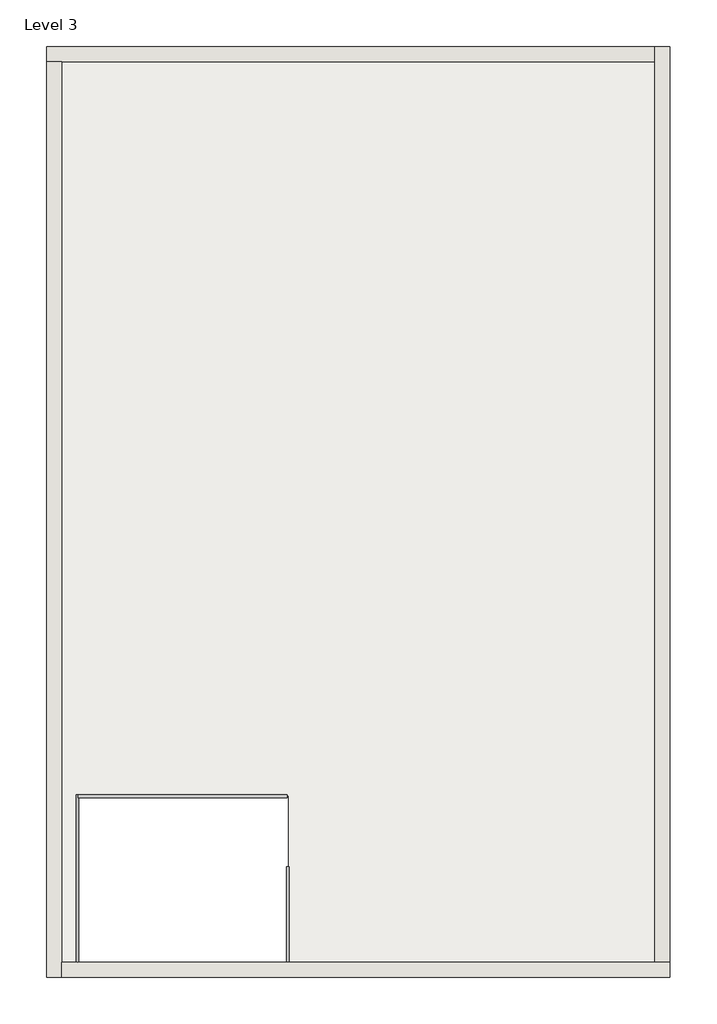
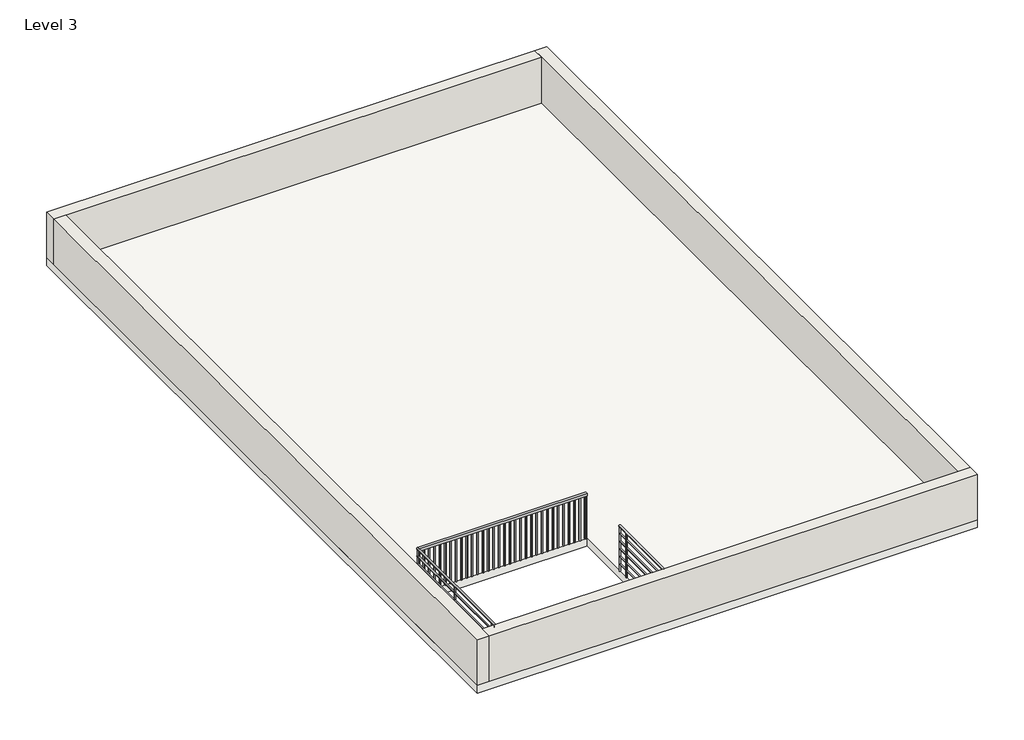
# One storey: 4 walls, 3 railings, 1 slab.
"""IFC4 building model written with IfcOpenShell, lengths in millimetres."""

from ifc_helpers import new_model, si_unit, point, frame, frame_2d, origin, place, context, project, spatial, polyline, circle_curve, trimmed, segment, composite_curve, outline, extrude, faceted_brep, element, save

model = new_model("IFC4")

# Units and contexts
model_context = context("Model", 3, world=origin())
ifc_project = project(units=[si_unit("LENGTHUNIT", "METRE", prefix="MILLI")], contexts=[model_context])

# Site, building, storey
site = spatial("IfcSite", under=ifc_project)
building = spatial("IfcBuilding", under=site)
storey = spatial("IfcBuildingStorey", under=building, Name="Level 3", Elevation=6400.8)

# Railings
placement = place(None, origin())
element("IfcRailing", 1, ObjectType="Handrail - Pipe", at=placement, inside=storey, context=model_context, shape_type="SweptSolid", body=[
    extrude(outline(composite_curve([segment(trimmed(circle_curve(frame_2d((7296.15, -11110.4683044)), 19.05), [point((7296.15, -11129.5183044))], [point((7296.15, -11091.4183044))], False, "CARTESIAN"), True, "CONTINUOUS"), segment(trimmed(circle_curve(frame_2d((7296.15, -11110.4683044)), 19.05), [point((7296.15, -11091.4183044))], [point((7296.15, -11129.5183044))], False, "CARTESIAN"), True, "CONTINUOUS")], self_intersect=False)), frame((0.0, -3889.1891189, 0.0), z_axis=(0.0, 1.0, 0.0), x_axis=(0.0, 0.0, 1.0)), (0.0, 0.0, 1.0), 2540.0),
    extrude(outline(composite_curve([segment(trimmed(circle_curve(frame_2d((7150.1, -11110.4683044)), 12.7), [point((7150.1, -11097.7683044))], [point((7150.1, -11123.1683044))], False, "CARTESIAN"), True, "CONTINUOUS"), segment(trimmed(circle_curve(frame_2d((7150.1, -11110.4683044)), 12.7), [point((7150.1, -11123.1683044))], [point((7150.1, -11097.7683044))], False, "CARTESIAN"), True, "CONTINUOUS")], self_intersect=False)), frame((0.0, -3889.1891189, 0.0), z_axis=(0.0, 1.0, 0.0), x_axis=(0.0, 0.0, 1.0)), (0.0, 0.0, 1.0), 2540.0),
    extrude(outline(composite_curve([segment(trimmed(circle_curve(frame_2d((6997.7, -11110.4683044)), 12.7), [point((6997.7, -11097.7683044))], [point((6997.7, -11123.1683044))], False, "CARTESIAN"), True, "CONTINUOUS"), segment(trimmed(circle_curve(frame_2d((6997.7, -11110.4683044)), 12.7), [point((6997.7, -11123.1683044))], [point((6997.7, -11097.7683044))], False, "CARTESIAN"), True, "CONTINUOUS")], self_intersect=False)), frame((0.0, -3889.1891189, 0.0), z_axis=(0.0, 1.0, 0.0), x_axis=(0.0, 0.0, 1.0)), (0.0, 0.0, 1.0), 2540.0),
    extrude(outline(composite_curve([segment(trimmed(circle_curve(frame_2d((6845.3, -11110.4683044)), 12.7), [point((6845.3, -11097.7683044))], [point((6845.3, -11123.1683044))], False, "CARTESIAN"), True, "CONTINUOUS"), segment(trimmed(circle_curve(frame_2d((6845.3, -11110.4683044)), 12.7), [point((6845.3, -11123.1683044))], [point((6845.3, -11097.7683044))], False, "CARTESIAN"), True, "CONTINUOUS")], self_intersect=False)), frame((0.0, -3889.1891189, 0.0), z_axis=(0.0, 1.0, 0.0), x_axis=(0.0, 0.0, 1.0)), (0.0, 0.0, 1.0), 2540.0),
    extrude(outline(composite_curve([segment(trimmed(circle_curve(frame_2d((6692.9, -11110.4683044)), 12.7), [point((6692.9, -11097.7683044))], [point((6692.9, -11123.1683044))], False, "CARTESIAN"), True, "CONTINUOUS"), segment(trimmed(circle_curve(frame_2d((6692.9, -11110.4683044)), 12.7), [point((6692.9, -11123.1683044))], [point((6692.9, -11097.7683044))], False, "CARTESIAN"), True, "CONTINUOUS")], self_intersect=False)), frame((0.0, -3889.1891189, 0.0), z_axis=(0.0, 1.0, 0.0), x_axis=(0.0, 0.0, 1.0)), (0.0, 0.0, 1.0), 2540.0),
    extrude(outline(composite_curve([segment(trimmed(circle_curve(frame_2d((6540.5, -11110.4683044)), 12.7), [point((6540.5, -11097.7683044))], [point((6540.5, -11123.1683044))], False, "CARTESIAN"), True, "CONTINUOUS"), segment(trimmed(circle_curve(frame_2d((6540.5, -11110.4683044)), 12.7), [point((6540.5, -11123.1683044))], [point((6540.5, -11097.7683044))], False, "CARTESIAN"), True, "CONTINUOUS")], self_intersect=False)), frame((0.0, -3889.1891189, 0.0), z_axis=(0.0, 1.0, 0.0), x_axis=(0.0, 0.0, 1.0)), (0.0, 0.0, 1.0), 2540.0),
    extrude(outline(composite_curve([segment(trimmed(circle_curve(frame_2d((-11110.4683044, -3787.5891189)), 12.7), [point((-11097.7683044, -3787.5891189))], [point((-11123.1683044, -3787.5891189))], False, "CARTESIAN"), True, "CONTINUOUS"), segment(trimmed(circle_curve(frame_2d((-11110.4683044, -3787.5891189)), 12.7), [point((-11123.1683044, -3787.5891189))], [point((-11097.7683044, -3787.5891189))], False, "CARTESIAN"), True, "CONTINUOUS")], self_intersect=False)), frame((0.0, 0.0, 6400.8), z_axis=(0.0, 0.0, 1.0), x_axis=(1.0, 0.0, 0.0)), (0.0, 0.0, 1.0), 876.3),
    extrude(outline(composite_curve([segment(trimmed(circle_curve(frame_2d((-11110.4683044, -2568.3891189)), 12.7), [point((-11097.7683044, -2568.3891189))], [point((-11123.1683044, -2568.3891189))], False, "CARTESIAN"), True, "CONTINUOUS"), segment(trimmed(circle_curve(frame_2d((-11110.4683044, -2568.3891189)), 12.7), [point((-11123.1683044, -2568.3891189))], [point((-11097.7683044, -2568.3891189))], False, "CARTESIAN"), True, "CONTINUOUS")], self_intersect=False)), frame((0.0, 0.0, 6400.8), z_axis=(0.0, 0.0, 1.0), x_axis=(1.0, 0.0, 0.0)), (0.0, 0.0, 1.0), 876.3),
    extrude(outline(composite_curve([segment(trimmed(circle_curve(frame_2d((-11110.4683044, -3876.4891189)), 12.7), [point((-11097.7683044, -3876.4891189))], [point((-11123.1683044, -3876.4891189))], False, "CARTESIAN"), True, "CONTINUOUS"), segment(trimmed(circle_curve(frame_2d((-11110.4683044, -3876.4891189)), 12.7), [point((-11123.1683044, -3876.4891189))], [point((-11097.7683044, -3876.4891189))], False, "CARTESIAN"), True, "CONTINUOUS")], self_intersect=False)), frame((0.0, 0.0, 6400.8), z_axis=(0.0, 0.0, 1.0), x_axis=(1.0, 0.0, 0.0)), (0.0, 0.0, 1.0), 876.3),
    extrude(outline(composite_curve([segment(trimmed(circle_curve(frame_2d((-11110.4683044, -1361.8891189)), 12.7), [point((-11097.7683044, -1361.8891189))], [point((-11123.1683044, -1361.8891189))], False, "CARTESIAN"), True, "CONTINUOUS"), segment(trimmed(circle_curve(frame_2d((-11110.4683044, -1361.8891189)), 12.7), [point((-11123.1683044, -1361.8891189))], [point((-11097.7683044, -1361.8891189))], False, "CARTESIAN"), True, "CONTINUOUS")], self_intersect=False)), frame((0.0, 0.0, 6400.8), z_axis=(0.0, 0.0, 1.0), x_axis=(1.0, 0.0, 0.0)), (0.0, 0.0, 1.0), 876.3),
])
element("IfcRailing", 2, ObjectType="Handrail - Pipe", at=placement, inside=storey, context=model_context, shape_type="SweptSolid", body=[
    extrude(outline(composite_curve([segment(trimmed(circle_curve(frame_2d((7296.15, -7922.7683044)), 19.05), [point((7296.15, -7903.7183044))], [point((7296.15, -7941.8183044))], False, "CARTESIAN"), True, "CONTINUOUS"), segment(trimmed(circle_curve(frame_2d((7296.15, -7922.7683044)), 19.05), [point((7296.15, -7941.8183044))], [point((7296.15, -7903.7183044))], False, "CARTESIAN"), True, "CONTINUOUS")], self_intersect=False)), frame((0.0, -3889.1891189, 0.0), z_axis=(0.0, 1.0, 0.0), x_axis=(0.0, 0.0, 1.0)), (0.0, 0.0, 1.0), 1447.8),
    extrude(outline(composite_curve([segment(trimmed(circle_curve(frame_2d((7150.1, -7922.7683044)), 12.7), [point((7150.1, -7935.4683044))], [point((7150.1, -7910.0683044))], False, "CARTESIAN"), True, "CONTINUOUS"), segment(trimmed(circle_curve(frame_2d((7150.1, -7922.7683044)), 12.7), [point((7150.1, -7910.0683044))], [point((7150.1, -7935.4683044))], False, "CARTESIAN"), True, "CONTINUOUS")], self_intersect=False)), frame((0.0, -3889.1891189, 0.0), z_axis=(0.0, 1.0, 0.0), x_axis=(0.0, 0.0, 1.0)), (0.0, 0.0, 1.0), 1447.8),
    extrude(outline(composite_curve([segment(trimmed(circle_curve(frame_2d((6997.7, -7922.7683044)), 12.7), [point((6997.7, -7935.4683044))], [point((6997.7, -7910.0683044))], False, "CARTESIAN"), True, "CONTINUOUS"), segment(trimmed(circle_curve(frame_2d((6997.7, -7922.7683044)), 12.7), [point((6997.7, -7910.0683044))], [point((6997.7, -7935.4683044))], False, "CARTESIAN"), True, "CONTINUOUS")], self_intersect=False)), frame((0.0, -3889.1891189, 0.0), z_axis=(0.0, 1.0, 0.0), x_axis=(0.0, 0.0, 1.0)), (0.0, 0.0, 1.0), 1447.8),
    extrude(outline(composite_curve([segment(trimmed(circle_curve(frame_2d((6845.3, -7922.7683044)), 12.7), [point((6845.3, -7935.4683044))], [point((6845.3, -7910.0683044))], False, "CARTESIAN"), True, "CONTINUOUS"), segment(trimmed(circle_curve(frame_2d((6845.3, -7922.7683044)), 12.7), [point((6845.3, -7910.0683044))], [point((6845.3, -7935.4683044))], False, "CARTESIAN"), True, "CONTINUOUS")], self_intersect=False)), frame((0.0, -3889.1891189, 0.0), z_axis=(0.0, 1.0, 0.0), x_axis=(0.0, 0.0, 1.0)), (0.0, 0.0, 1.0), 1447.8),
    extrude(outline(composite_curve([segment(trimmed(circle_curve(frame_2d((6692.9, -7922.7683044)), 12.7), [point((6692.9, -7935.4683044))], [point((6692.9, -7910.0683044))], False, "CARTESIAN"), True, "CONTINUOUS"), segment(trimmed(circle_curve(frame_2d((6692.9, -7922.7683044)), 12.7), [point((6692.9, -7910.0683044))], [point((6692.9, -7935.4683044))], False, "CARTESIAN"), True, "CONTINUOUS")], self_intersect=False)), frame((0.0, -3889.1891189, 0.0), z_axis=(0.0, 1.0, 0.0), x_axis=(0.0, 0.0, 1.0)), (0.0, 0.0, 1.0), 1447.8),
    extrude(outline(composite_curve([segment(trimmed(circle_curve(frame_2d((6540.5, -7922.7683044)), 12.7), [point((6540.5, -7935.4683044))], [point((6540.5, -7910.0683044))], False, "CARTESIAN"), True, "CONTINUOUS"), segment(trimmed(circle_curve(frame_2d((6540.5, -7922.7683044)), 12.7), [point((6540.5, -7910.0683044))], [point((6540.5, -7935.4683044))], False, "CARTESIAN"), True, "CONTINUOUS")], self_intersect=False)), frame((0.0, -3889.1891189, 0.0), z_axis=(0.0, 1.0, 0.0), x_axis=(0.0, 0.0, 1.0)), (0.0, 0.0, 1.0), 1447.8),
    extrude(outline(composite_curve([segment(trimmed(circle_curve(frame_2d((-7922.7683044, -2669.9891189)), 12.7), [point((-7935.4683044, -2669.9891189))], [point((-7910.0683044, -2669.9891189))], False, "CARTESIAN"), True, "CONTINUOUS"), segment(trimmed(circle_curve(frame_2d((-7922.7683044, -2669.9891189)), 12.7), [point((-7910.0683044, -2669.9891189))], [point((-7935.4683044, -2669.9891189))], False, "CARTESIAN"), True, "CONTINUOUS")], self_intersect=False)), frame((0.0, 0.0, 6400.8), z_axis=(0.0, 0.0, 1.0), x_axis=(1.0, 0.0, 0.0)), (0.0, 0.0, 1.0), 876.3),
    extrude(outline(composite_curve([segment(trimmed(circle_curve(frame_2d((-7922.7683044, -2454.0891189)), 12.7), [point((-7935.4683044, -2454.0891189))], [point((-7910.0683044, -2454.0891189))], False, "CARTESIAN"), True, "CONTINUOUS"), segment(trimmed(circle_curve(frame_2d((-7922.7683044, -2454.0891189)), 12.7), [point((-7910.0683044, -2454.0891189))], [point((-7935.4683044, -2454.0891189))], False, "CARTESIAN"), True, "CONTINUOUS")], self_intersect=False)), frame((0.0, 0.0, 6400.8), z_axis=(0.0, 0.0, 1.0), x_axis=(1.0, 0.0, 0.0)), (0.0, 0.0, 1.0), 876.3),
    extrude(outline(composite_curve([segment(trimmed(circle_curve(frame_2d((-7922.7683044, -3876.4891189)), 12.7), [point((-7935.4683044, -3876.4891189))], [point((-7910.0683044, -3876.4891189))], False, "CARTESIAN"), True, "CONTINUOUS"), segment(trimmed(circle_curve(frame_2d((-7922.7683044, -3876.4891189)), 12.7), [point((-7910.0683044, -3876.4891189))], [point((-7935.4683044, -3876.4891189))], False, "CARTESIAN"), True, "CONTINUOUS")], self_intersect=False)), frame((0.0, 0.0, 6400.8), z_axis=(0.0, 0.0, 1.0), x_axis=(1.0, 0.0, 0.0)), (0.0, 0.0, 1.0), 876.3),
])
element("IfcRailing", 3, ObjectType="Handrail - Rectangular", at=placement, inside=storey, context=model_context, shape_type="SweptSolid", body=[
    extrude(outline(polyline([(-11110.4683044, -1399.9891189), (-11110.4683044, -1349.1891189), (-7935.4683044, -1349.1891189), (-7935.4683044, -1399.9891189), (-11110.4683044, -1399.9891189)])), frame((0.0, 0.0, 7264.4), z_axis=(0.0, 0.0, 1.0), x_axis=(1.0, 0.0, 0.0)), (0.0, 0.0, 1.0), 50.8),
    extrude(outline(polyline([(-7970.3933044, -1384.1141189), (-7970.3933044, -1365.0641189), (-7951.3433044, -1365.0641189), (-7951.3433044, -1384.1141189), (-7970.3933044, -1384.1141189)])), frame((0.0, 0.0, 6400.8), z_axis=(0.0, 0.0, 1.0), x_axis=(1.0, 0.0, 0.0)), (0.0, 0.0, 1.0), 863.6),
    extrude(outline(polyline([(-8071.9933044, -1384.1141189), (-8071.9933044, -1365.0641189), (-8052.9433044, -1365.0641189), (-8052.9433044, -1384.1141189), (-8071.9933044, -1384.1141189)])), frame((0.0, 0.0, 6400.8), z_axis=(0.0, 0.0, 1.0), x_axis=(1.0, 0.0, 0.0)), (0.0, 0.0, 1.0), 863.6),
    extrude(outline(polyline([(-8173.5933044, -1384.1141189), (-8173.5933044, -1365.0641189), (-8154.5433044, -1365.0641189), (-8154.5433044, -1384.1141189), (-8173.5933044, -1384.1141189)])), frame((0.0, 0.0, 6400.8), z_axis=(0.0, 0.0, 1.0), x_axis=(1.0, 0.0, 0.0)), (0.0, 0.0, 1.0), 863.6),
    extrude(outline(polyline([(-8275.1933044, -1384.1141189), (-8275.1933044, -1365.0641189), (-8256.1433044, -1365.0641189), (-8256.1433044, -1384.1141189), (-8275.1933044, -1384.1141189)])), frame((0.0, 0.0, 6400.8), z_axis=(0.0, 0.0, 1.0), x_axis=(1.0, 0.0, 0.0)), (0.0, 0.0, 1.0), 863.6),
    extrude(outline(polyline([(-8376.7933044, -1384.1141189), (-8376.7933044, -1365.0641189), (-8357.7433044, -1365.0641189), (-8357.7433044, -1384.1141189), (-8376.7933044, -1384.1141189)])), frame((0.0, 0.0, 6400.8), z_axis=(0.0, 0.0, 1.0), x_axis=(1.0, 0.0, 0.0)), (0.0, 0.0, 1.0), 863.6),
    extrude(outline(polyline([(-8478.3933044, -1384.1141189), (-8478.3933044, -1365.0641189), (-8459.3433044, -1365.0641189), (-8459.3433044, -1384.1141189), (-8478.3933044, -1384.1141189)])), frame((0.0, 0.0, 6400.8), z_axis=(0.0, 0.0, 1.0), x_axis=(1.0, 0.0, 0.0)), (0.0, 0.0, 1.0), 863.6),
    extrude(outline(polyline([(-8579.9933044, -1384.1141189), (-8579.9933044, -1365.0641189), (-8560.9433044, -1365.0641189), (-8560.9433044, -1384.1141189), (-8579.9933044, -1384.1141189)])), frame((0.0, 0.0, 6400.8), z_axis=(0.0, 0.0, 1.0), x_axis=(1.0, 0.0, 0.0)), (0.0, 0.0, 1.0), 863.6),
    extrude(outline(polyline([(-8681.5933044, -1384.1141189), (-8681.5933044, -1365.0641189), (-8662.5433044, -1365.0641189), (-8662.5433044, -1384.1141189), (-8681.5933044, -1384.1141189)])), frame((0.0, 0.0, 6400.8), z_axis=(0.0, 0.0, 1.0), x_axis=(1.0, 0.0, 0.0)), (0.0, 0.0, 1.0), 863.6),
    extrude(outline(polyline([(-8783.1933044, -1384.1141189), (-8783.1933044, -1365.0641189), (-8764.1433044, -1365.0641189), (-8764.1433044, -1384.1141189), (-8783.1933044, -1384.1141189)])), frame((0.0, 0.0, 6400.8), z_axis=(0.0, 0.0, 1.0), x_axis=(1.0, 0.0, 0.0)), (0.0, 0.0, 1.0), 863.6),
    extrude(outline(polyline([(-8884.7933044, -1384.1141189), (-8884.7933044, -1365.0641189), (-8865.7433044, -1365.0641189), (-8865.7433044, -1384.1141189), (-8884.7933044, -1384.1141189)])), frame((0.0, 0.0, 6400.8), z_axis=(0.0, 0.0, 1.0), x_axis=(1.0, 0.0, 0.0)), (0.0, 0.0, 1.0), 863.6),
    extrude(outline(polyline([(-8986.3933044, -1384.1141189), (-8986.3933044, -1365.0641189), (-8967.3433044, -1365.0641189), (-8967.3433044, -1384.1141189), (-8986.3933044, -1384.1141189)])), frame((0.0, 0.0, 6400.8), z_axis=(0.0, 0.0, 1.0), x_axis=(1.0, 0.0, 0.0)), (0.0, 0.0, 1.0), 863.6),
    extrude(outline(polyline([(-9087.9933044, -1384.1141189), (-9087.9933044, -1365.0641189), (-9068.9433044, -1365.0641189), (-9068.9433044, -1384.1141189), (-9087.9933044, -1384.1141189)])), frame((0.0, 0.0, 6400.8), z_axis=(0.0, 0.0, 1.0), x_axis=(1.0, 0.0, 0.0)), (0.0, 0.0, 1.0), 863.6),
    extrude(outline(polyline([(-9189.5933044, -1384.1141189), (-9189.5933044, -1365.0641189), (-9170.5433044, -1365.0641189), (-9170.5433044, -1384.1141189), (-9189.5933044, -1384.1141189)])), frame((0.0, 0.0, 6400.8), z_axis=(0.0, 0.0, 1.0), x_axis=(1.0, 0.0, 0.0)), (0.0, 0.0, 1.0), 863.6),
    extrude(outline(polyline([(-9291.1933044, -1384.1141189), (-9291.1933044, -1365.0641189), (-9272.1433044, -1365.0641189), (-9272.1433044, -1384.1141189), (-9291.1933044, -1384.1141189)])), frame((0.0, 0.0, 6400.8), z_axis=(0.0, 0.0, 1.0), x_axis=(1.0, 0.0, 0.0)), (0.0, 0.0, 1.0), 863.6),
    extrude(outline(polyline([(-9392.7933044, -1384.1141189), (-9392.7933044, -1365.0641189), (-9373.7433044, -1365.0641189), (-9373.7433044, -1384.1141189), (-9392.7933044, -1384.1141189)])), frame((0.0, 0.0, 6400.8), z_axis=(0.0, 0.0, 1.0), x_axis=(1.0, 0.0, 0.0)), (0.0, 0.0, 1.0), 863.6),
    extrude(outline(polyline([(-9494.3933044, -1384.1141189), (-9494.3933044, -1365.0641189), (-9475.3433044, -1365.0641189), (-9475.3433044, -1384.1141189), (-9494.3933044, -1384.1141189)])), frame((0.0, 0.0, 6400.8), z_axis=(0.0, 0.0, 1.0), x_axis=(1.0, 0.0, 0.0)), (0.0, 0.0, 1.0), 863.6),
    extrude(outline(polyline([(-9595.9933044, -1384.1141189), (-9595.9933044, -1365.0641189), (-9576.9433044, -1365.0641189), (-9576.9433044, -1384.1141189), (-9595.9933044, -1384.1141189)])), frame((0.0, 0.0, 6400.8), z_axis=(0.0, 0.0, 1.0), x_axis=(1.0, 0.0, 0.0)), (0.0, 0.0, 1.0), 863.6),
    extrude(outline(polyline([(-9697.5933044, -1384.1141189), (-9697.5933044, -1365.0641189), (-9678.5433044, -1365.0641189), (-9678.5433044, -1384.1141189), (-9697.5933044, -1384.1141189)])), frame((0.0, 0.0, 6400.8), z_axis=(0.0, 0.0, 1.0), x_axis=(1.0, 0.0, 0.0)), (0.0, 0.0, 1.0), 863.6),
    extrude(outline(polyline([(-9799.1933044, -1384.1141189), (-9799.1933044, -1365.0641189), (-9780.1433044, -1365.0641189), (-9780.1433044, -1384.1141189), (-9799.1933044, -1384.1141189)])), frame((0.0, 0.0, 6400.8), z_axis=(0.0, 0.0, 1.0), x_axis=(1.0, 0.0, 0.0)), (0.0, 0.0, 1.0), 863.6),
    extrude(outline(polyline([(-9900.7933044, -1384.1141189), (-9900.7933044, -1365.0641189), (-9881.7433044, -1365.0641189), (-9881.7433044, -1384.1141189), (-9900.7933044, -1384.1141189)])), frame((0.0, 0.0, 6400.8), z_axis=(0.0, 0.0, 1.0), x_axis=(1.0, 0.0, 0.0)), (0.0, 0.0, 1.0), 863.6),
    extrude(outline(polyline([(-10002.3933044, -1384.1141189), (-10002.3933044, -1365.0641189), (-9983.3433044, -1365.0641189), (-9983.3433044, -1384.1141189), (-10002.3933044, -1384.1141189)])), frame((0.0, 0.0, 6400.8), z_axis=(0.0, 0.0, 1.0), x_axis=(1.0, 0.0, 0.0)), (0.0, 0.0, 1.0), 863.6),
    extrude(outline(polyline([(-10103.9933044, -1384.1141189), (-10103.9933044, -1365.0641189), (-10084.9433044, -1365.0641189), (-10084.9433044, -1384.1141189), (-10103.9933044, -1384.1141189)])), frame((0.0, 0.0, 6400.8), z_axis=(0.0, 0.0, 1.0), x_axis=(1.0, 0.0, 0.0)), (0.0, 0.0, 1.0), 863.6),
    extrude(outline(polyline([(-10205.5933044, -1384.1141189), (-10205.5933044, -1365.0641189), (-10186.5433044, -1365.0641189), (-10186.5433044, -1384.1141189), (-10205.5933044, -1384.1141189)])), frame((0.0, 0.0, 6400.8), z_axis=(0.0, 0.0, 1.0), x_axis=(1.0, 0.0, 0.0)), (0.0, 0.0, 1.0), 863.6),
    extrude(outline(polyline([(-10307.1933044, -1384.1141189), (-10307.1933044, -1365.0641189), (-10288.1433044, -1365.0641189), (-10288.1433044, -1384.1141189), (-10307.1933044, -1384.1141189)])), frame((0.0, 0.0, 6400.8), z_axis=(0.0, 0.0, 1.0), x_axis=(1.0, 0.0, 0.0)), (0.0, 0.0, 1.0), 863.6),
    extrude(outline(polyline([(-10408.7933044, -1384.1141189), (-10408.7933044, -1365.0641189), (-10389.7433044, -1365.0641189), (-10389.7433044, -1384.1141189), (-10408.7933044, -1384.1141189)])), frame((0.0, 0.0, 6400.8), z_axis=(0.0, 0.0, 1.0), x_axis=(1.0, 0.0, 0.0)), (0.0, 0.0, 1.0), 863.6),
    extrude(outline(polyline([(-10510.3933044, -1384.1141189), (-10510.3933044, -1365.0641189), (-10491.3433044, -1365.0641189), (-10491.3433044, -1384.1141189), (-10510.3933044, -1384.1141189)])), frame((0.0, 0.0, 6400.8), z_axis=(0.0, 0.0, 1.0), x_axis=(1.0, 0.0, 0.0)), (0.0, 0.0, 1.0), 863.6),
    extrude(outline(polyline([(-10611.9933044, -1384.1141189), (-10611.9933044, -1365.0641189), (-10592.9433044, -1365.0641189), (-10592.9433044, -1384.1141189), (-10611.9933044, -1384.1141189)])), frame((0.0, 0.0, 6400.8), z_axis=(0.0, 0.0, 1.0), x_axis=(1.0, 0.0, 0.0)), (0.0, 0.0, 1.0), 863.6),
    extrude(outline(polyline([(-10713.5933044, -1384.1141189), (-10713.5933044, -1365.0641189), (-10694.5433044, -1365.0641189), (-10694.5433044, -1384.1141189), (-10713.5933044, -1384.1141189)])), frame((0.0, 0.0, 6400.8), z_axis=(0.0, 0.0, 1.0), x_axis=(1.0, 0.0, 0.0)), (0.0, 0.0, 1.0), 863.6),
    extrude(outline(polyline([(-10815.1933044, -1384.1141189), (-10815.1933044, -1365.0641189), (-10796.1433044, -1365.0641189), (-10796.1433044, -1384.1141189), (-10815.1933044, -1384.1141189)])), frame((0.0, 0.0, 6400.8), z_axis=(0.0, 0.0, 1.0), x_axis=(1.0, 0.0, 0.0)), (0.0, 0.0, 1.0), 863.6),
    extrude(outline(polyline([(-10916.7933044, -1384.1141189), (-10916.7933044, -1365.0641189), (-10897.7433044, -1365.0641189), (-10897.7433044, -1384.1141189), (-10916.7933044, -1384.1141189)])), frame((0.0, 0.0, 6400.8), z_axis=(0.0, 0.0, 1.0), x_axis=(1.0, 0.0, 0.0)), (0.0, 0.0, 1.0), 863.6),
    extrude(outline(polyline([(-11018.3933044, -1384.1141189), (-11018.3933044, -1365.0641189), (-10999.3433044, -1365.0641189), (-10999.3433044, -1384.1141189), (-11018.3933044, -1384.1141189)])), frame((0.0, 0.0, 6400.8), z_axis=(0.0, 0.0, 1.0), x_axis=(1.0, 0.0, 0.0)), (0.0, 0.0, 1.0), 863.6),
    extrude(outline(polyline([(-7954.5183044, -1384.1141189), (-7954.5183044, -1365.0641189), (-7935.4683044, -1365.0641189), (-7935.4683044, -1384.1141189), (-7954.5183044, -1384.1141189)])), frame((0.0, 0.0, 6400.8), z_axis=(0.0, 0.0, 1.0), x_axis=(1.0, 0.0, 0.0)), (0.0, 0.0, 1.0), 863.6),
    extrude(outline(polyline([(-11110.4683044, -1384.1141189), (-11110.4683044, -1365.0641189), (-11091.4183044, -1365.0641189), (-11091.4183044, -1384.1141189), (-11110.4683044, -1384.1141189)])), frame((0.0, 0.0, 6400.8), z_axis=(0.0, 0.0, 1.0), x_axis=(1.0, 0.0, 0.0)), (0.0, 0.0, 1.0), 863.6),
])

# Slab
element("IfcSlab", 4, ObjectType="6\"", at=placement, inside=storey, context=model_context, shape_type="SweptSolid", body=[
    extrude(outline(polyline([(-2131.5683044, 9979.2108811), (-2131.5683044, -4117.7891189), (-11580.3683044, -4117.7891189), (-11580.3683044, 9979.2108811), (-2131.5683044, 9979.2108811)]), holes=[polyline([(-7922.7683044, -1374.5891189), (-11110.4683044, -1374.5891189), (-11110.4683044, -3889.1891189), (-7922.7683044, -3889.1891189), (-7922.7683044, -1374.5891189)])]), frame((0.0, 0.0, 6248.4), z_axis=(0.0, 0.0, 1.0), x_axis=(1.0, 0.0, 0.0)), (0.0, 0.0, 1.0), 152.4),
])

# Walls
element("IfcWall", 5, ObjectType="9\"", at=placement, inside=storey, context=model_context, shape_type="Brep", body=[
    faceted_brep([(-11580.3683044, 9750.6108811, 6400.8), (-11351.7683044, 9750.6108811, 6400.8), (-2360.1683044, 9750.6108811, 6400.8), (-2360.1683044, 9750.6108811, 7315.2), (-11351.7683044, 9750.6108811, 7315.2), (-11580.3683044, 9750.6108811, 7315.2), (-11580.3683044, 9979.2108811, 6400.8), (-11580.3683044, 9979.2108811, 7315.2), (-2360.1683044, 9979.2108811, 7315.2), (-2360.1683044, 9979.2108811, 6400.8)], [[[0, 1, 2, 3, 4, 5]], [[6, 7, 8, 9]], [[2, 1, 0, 6, 9]], [[5, 4, 3, 8, 7]], [[0, 5, 7, 6]], [[3, 2, 9, 8]]]),
])
element("IfcWall", 6, ObjectType="9\"", at=placement, inside=storey, context=model_context, shape_type="Brep", body=[
    faceted_brep([(-11351.7683044, -4117.7891189, 6400.8), (-11351.7683044, -3889.1891189, 6400.8), (-11351.7683044, 9750.6108811, 6400.8), (-11351.7683044, 9750.6108811, 7315.2), (-11351.7683044, -3889.1891189, 7315.2), (-11351.7683044, -4117.7891189, 7315.2), (-11580.3683044, -4117.7891189, 6400.8), (-11580.3683044, -4117.7891189, 7315.2), (-11580.3683044, 9750.6108811, 7315.2), (-11580.3683044, 9750.6108811, 6400.8)], [[[0, 1, 2, 3, 4, 5]], [[6, 7, 8, 9]], [[2, 1, 0, 6, 9]], [[5, 4, 3, 8, 7]], [[0, 5, 7, 6]], [[3, 2, 9, 8]]]),
])
element("IfcWall", 7, ObjectType="9\"", at=placement, inside=storey, context=model_context, shape_type="Brep", body=[
    faceted_brep([(-2131.5683044, -3889.1891189, 6400.8), (-2360.1683044, -3889.1891189, 6400.8), (-11351.7683044, -3889.1891189, 6400.8), (-11351.7683044, -3889.1891189, 7315.2), (-2360.1683044, -3889.1891189, 7315.2), (-2131.5683044, -3889.1891189, 7315.2), (-2131.5683044, -4117.7891189, 6400.8), (-2131.5683044, -4117.7891189, 7315.2), (-11351.7683044, -4117.7891189, 7315.2), (-11351.7683044, -4117.7891189, 6400.8)], [[[0, 1, 2, 3, 4, 5]], [[6, 7, 8, 9]], [[2, 1, 0, 6, 9]], [[5, 4, 3, 8, 7]], [[0, 5, 7, 6]], [[3, 2, 9, 8]]]),
])
element("IfcWall", 8, ObjectType="9\"", at=placement, inside=storey, context=model_context, shape_type="Brep", body=[
    faceted_brep([(-2360.1683044, 9979.2108811, 6400.8), (-2360.1683044, 9750.6108811, 6400.8), (-2360.1683044, -3889.1891189, 6400.8), (-2360.1683044, -3889.1891189, 7315.2), (-2360.1683044, 9750.6108811, 7315.2), (-2360.1683044, 9979.2108811, 7315.2), (-2131.5683044, 9979.2108811, 6400.8), (-2131.5683044, 9979.2108811, 7315.2), (-2131.5683044, -3889.1891189, 7315.2), (-2131.5683044, -3889.1891189, 6400.8)], [[[0, 1, 2, 3, 4, 5]], [[6, 7, 8, 9]], [[2, 1, 0, 6, 9]], [[5, 4, 3, 8, 7]], [[0, 5, 7, 6]], [[3, 2, 9, 8]]]),
])

save(model, "model.ifc")

# Revit data of these elements
# Type "Handrail - Pipe"
#   Assembly Code = "C2010400"
#   built-in parameter 1008612 = 0.0416667 (stored number, unit not read)
#   built-in parameter 1008611 = 0.0833333 (stored number, unit not read)
#   built-in parameter 1008609 = 4 (stored number, unit not read)
#   built-in parameter 1008604 = 0.166667 (stored number, unit not read)
#   built-in parameter 1008603 = 0.166667 (stored number, unit not read)
#   Railing Height = 3' - 0"
#   built-in parameter 1008630 = 2
#   built-in parameter 1008610 = 1
#   built-in parameter 1008605 = 1
#   built-in parameter 1008618 = Baluster - Round : 1"
# Type "Handrail - Rectangular"
#   Assembly Code = "C2010400"
#   built-in parameter 1008612 = 0.0416667 (stored number, unit not read)
#   built-in parameter 1008611 = 0.0416667 (stored number, unit not read)
#   built-in parameter 1008609 = 0.333333 (stored number, unit not read)
#   built-in parameter 1008604 = 0.166667 (stored number, unit not read)
#   built-in parameter 1008603 = 0.166667 (stored number, unit not read)
#   Railing Height = 3' - 0"
#   built-in parameter 1008630 = 2
#   built-in parameter 1008610 = 2
#   built-in parameter 1008618 = Baluster - Square : 3/4"
# Type "6\""
#   Assembly Code = "B1010"
#   Function = 0
#   Layers, outside or top first: 0' - 6" "floor" (function 1)
# Type "9\""
#   Assembly Code = "B2010"
#   Layers, outside or top first: 0' - 9" "ext wall" (function 1)
# Elements 1, 2 (IfcRailing, "Handrail - Pipe")
#   Phase Created = New Construction
# Element 3 (IfcRailing, "Handrail - Rectangular")
#   Phase Created = New Construction
# Element 4 (IfcSlab, "6\"")
#   Height Offset From Level = 0' - 0"
#   Phase Created = New Construction
#   Materials on its faces: "floor"
# Elements 5, 6, 7, 8 (IfcWall, "9\"")
#   Top Offset = 0' - 0"
#   Base Offset = 0' - 0"
#   Unconnected Height = 3' - 0"
#   wall height = 3' - 0"
#   Phase Created = New Construction
#   Base Constraint = Level 3
#   Materials on its faces: "ext wall"
# Materials
#   "floor": class "Generic", colour RGB 146 137 125, transparency 0, Cost = 0
#   "ext wall": class "Generic", colour RGB 230 213 172, transparency 0, Cost = 0
